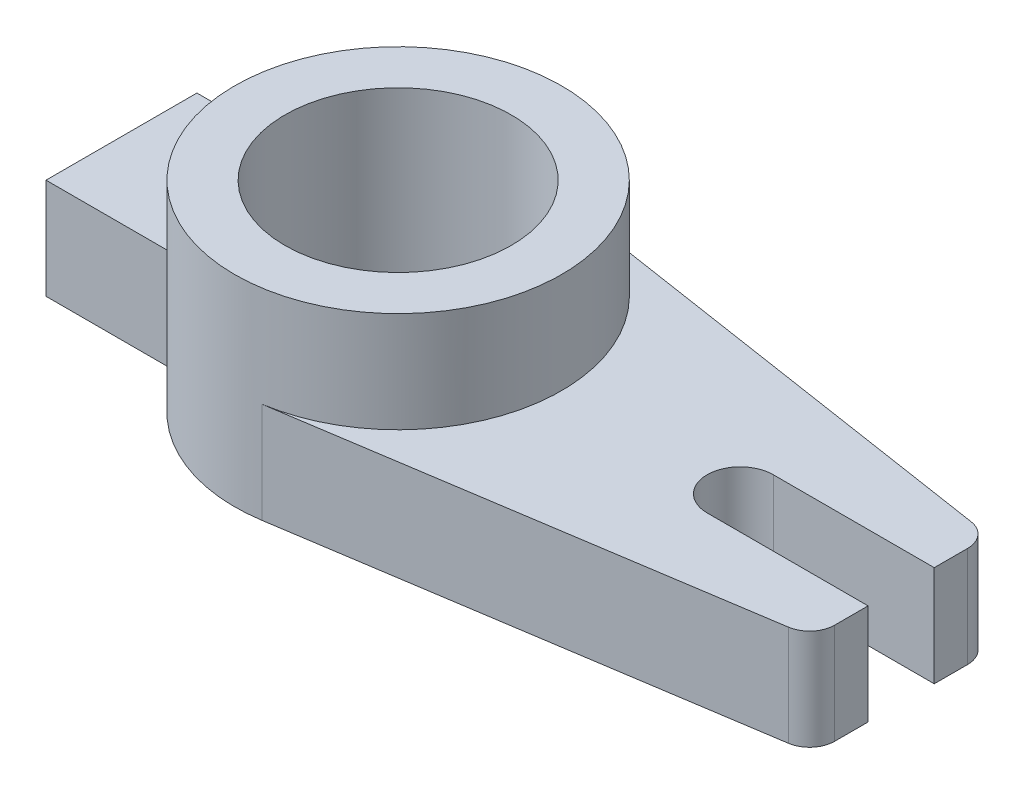
ISO-10303-21;
HEADER;
FILE_DESCRIPTION(('STEP AP214'),'2;1');
FILE_NAME('part.step','',(''),(''),'','','');
FILE_SCHEMA(('AUTOMOTIVE_DESIGN { 1 0 10303 214 1 1 1 1 }'));
ENDSEC;
DATA;
#1=APPLICATION_CONTEXT('core data for automotive mechanical design processes');
#2=APPLICATION_PROTOCOL_DEFINITION('international standard','automotive_design',2000,#1);
#3=PRODUCT_CONTEXT('',#1,'mechanical');
#4=PRODUCT('Part','Part','',(#3));
#5=PRODUCT_RELATED_PRODUCT_CATEGORY('part','',(#4));
#6=PRODUCT_DEFINITION_FORMATION('','',#4);
#7=PRODUCT_DEFINITION_CONTEXT('part definition',#1,'design');
#8=PRODUCT_DEFINITION('design','',#6,#7);
#9=PRODUCT_DEFINITION_SHAPE('','',#8);
#10=(LENGTH_UNIT() NAMED_UNIT(*) SI_UNIT(.MILLI.,.METRE.));
#11=(NAMED_UNIT(*) PLANE_ANGLE_UNIT() SI_UNIT($,.RADIAN.));
#12=(NAMED_UNIT(*) SI_UNIT($,.STERADIAN.) SOLID_ANGLE_UNIT());
#13=UNCERTAINTY_MEASURE_WITH_UNIT(LENGTH_MEASURE(1.E-05),#10,'distance_accuracy_value','');
#14=(GEOMETRIC_REPRESENTATION_CONTEXT(3) GLOBAL_UNCERTAINTY_ASSIGNED_CONTEXT((#13)) GLOBAL_UNIT_ASSIGNED_CONTEXT((#10,
#11,#12)) REPRESENTATION_CONTEXT('',''));
#15=CARTESIAN_POINT('',(0.,0.,0.));
#16=DIRECTION('',(0.,0.,1.));
#17=DIRECTION('',(1.,0.,0.));
#18=AXIS2_PLACEMENT_3D('',#15,#16,#17);
#19=CARTESIAN_POINT('',(0.,40.,0.));
#20=DIRECTION('',(0.,-1.,0.));
#21=DIRECTION('',(0.,0.,-1.));
#22=AXIS2_PLACEMENT_3D('',#19,#20,#21);
#23=CYLINDRICAL_SURFACE('',#22,32.5);
#24=CARTESIAN_POINT('',(0.,40.,0.));
#25=DIRECTION('',(0.,1.,0.));
#26=DIRECTION('',(0.,0.,1.));
#27=AXIS2_PLACEMENT_3D('',#24,#25,#26);
#28=CIRCLE('',#27,32.5);
#29=CARTESIAN_POINT('',(0.,40.,32.5));
#30=VERTEX_POINT('',#29);
#31=EDGE_CURVE('E11',#30,#30,#28,.T.);
#32=ORIENTED_EDGE('',*,*,#31,.F.);
#33=EDGE_LOOP('',(#32));
#34=FACE_BOUND('',#33,.T.);
#35=DIRECTION('',(0.,-1.,0.));
#36=VECTOR('',#35,1.);
#37=CARTESIAN_POINT('',(-28.831406486677,20.,-15.));
#38=LINE('',#37,#36);
#39=CARTESIAN_POINT('',(-28.831406486677,20.,-15.));
#40=VERTEX_POINT('',#39);
#41=CARTESIAN_POINT('',(-28.831406486677,0.,-15.));
#42=VERTEX_POINT('',#41);
#43=EDGE_CURVE('E59',#40,#42,#38,.T.);
#44=ORIENTED_EDGE('',*,*,#43,.F.);
#45=CARTESIAN_POINT('',(0.,20.,0.));
#46=DIRECTION('',(0.,-1.,0.));
#47=DIRECTION('',(0.,0.,1.));
#48=AXIS2_PLACEMENT_3D('',#45,#46,#47);
#49=CIRCLE('',#48,32.5);
#50=CARTESIAN_POINT('',(-28.831406486677,20.,15.));
#51=VERTEX_POINT('',#50);
#52=EDGE_CURVE('E52',#51,#40,#49,.T.);
#53=ORIENTED_EDGE('',*,*,#52,.F.);
#54=DIRECTION('',(0.,-1.,0.));
#55=VECTOR('',#54,1.);
#56=CARTESIAN_POINT('',(-28.831406486677,20.,15.));
#57=LINE('',#56,#55);
#58=CARTESIAN_POINT('',(-28.831406486677,0.,15.));
#59=VERTEX_POINT('',#58);
#60=EDGE_CURVE('E163',#51,#59,#57,.T.);
#61=ORIENTED_EDGE('',*,*,#60,.T.);
#62=CARTESIAN_POINT('',(0.,0.,0.));
#63=DIRECTION('',(0.,1.,0.));
#64=DIRECTION('',(0.,0.,1.));
#65=AXIS2_PLACEMENT_3D('',#62,#63,#64);
#66=CIRCLE('',#65,32.5);
#67=CARTESIAN_POINT('',(5.0678114160152,0.,32.1024498668202));
#68=VERTEX_POINT('',#67);
#69=EDGE_CURVE('E243',#59,#68,#66,.T.);
#70=ORIENTED_EDGE('',*,*,#69,.T.);
#71=DIRECTION('',(0.,-1.,0.));
#72=VECTOR('',#71,1.);
#73=CARTESIAN_POINT('',(5.06781141601827,20.,32.1024498668198));
#74=LINE('',#73,#72);
#75=CARTESIAN_POINT('',(5.06781141601827,20.,32.1024498668197));
#76=VERTEX_POINT('',#75);
#77=EDGE_CURVE('E218',#76,#68,#74,.T.);
#78=ORIENTED_EDGE('',*,*,#77,.F.);
#79=CARTESIAN_POINT('',(0.,20.,0.));
#80=DIRECTION('',(0.,-1.,0.));
#81=DIRECTION('',(0.,0.,1.));
#82=AXIS2_PLACEMENT_3D('',#79,#80,#81);
#83=CIRCLE('',#82,32.5);
#84=CARTESIAN_POINT('',(5.0678114160152,20.,-32.1024498668202));
#85=VERTEX_POINT('',#84);
#86=EDGE_CURVE('E182',#85,#76,#83,.T.);
#87=ORIENTED_EDGE('',*,*,#86,.F.);
#88=DIRECTION('',(0.,-1.,0.));
#89=VECTOR('',#88,1.);
#90=CARTESIAN_POINT('',(5.06781141601827,20.,-32.1024498668198));
#91=LINE('',#90,#89);
#92=CARTESIAN_POINT('',(5.06781141601827,0.,-32.1024498668198));
#93=VERTEX_POINT('',#92);
#94=EDGE_CURVE('E225',#85,#93,#91,.T.);
#95=ORIENTED_EDGE('',*,*,#94,.T.);
#96=EDGE_CURVE('E45',#93,#42,#66,.T.);
#97=ORIENTED_EDGE('',*,*,#96,.T.);
#98=EDGE_LOOP('',(#44,#53,#61,#70,#78,#87,#95,#97));
#99=FACE_BOUND('',#98,.T.);
#100=ADVANCED_FACE('F39',(#34,#99),#23,.T.);
#101=CARTESIAN_POINT('',(0.,40.,0.));
#102=DIRECTION('',(0.,1.,0.));
#103=DIRECTION('',(0.,0.,1.));
#104=AXIS2_PLACEMENT_3D('',#101,#102,#103);
#105=PLANE('',#104);
#106=ORIENTED_EDGE('',*,*,#31,.T.);
#107=EDGE_LOOP('',(#106));
#108=FACE_BOUND('',#107,.T.);
#109=CARTESIAN_POINT('',(0.,40.,0.));
#110=DIRECTION('',(0.,1.,0.));
#111=DIRECTION('',(0.,0.,1.));
#112=AXIS2_PLACEMENT_3D('',#109,#110,#111);
#113=CIRCLE('',#112,22.5);
#114=CARTESIAN_POINT('',(0.,40.,22.5));
#115=VERTEX_POINT('',#114);
#116=EDGE_CURVE('E236',#115,#115,#113,.T.);
#117=ORIENTED_EDGE('',*,*,#116,.F.);
#118=EDGE_LOOP('',(#117));
#119=FACE_BOUND('',#118,.T.);
#120=ADVANCED_FACE('F257',(#108,#119),#105,.T.);
#121=CARTESIAN_POINT('',(0.,0.,0.));
#122=DIRECTION('',(0.,1.,0.));
#123=DIRECTION('',(0.,0.,1.));
#124=AXIS2_PLACEMENT_3D('',#121,#122,#123);
#125=PLANE('',#124);
#126=ORIENTED_EDGE('',*,*,#96,.F.);
#127=DIRECTION('',(-0.988375612593621,0.,-0.152031734944335));
#128=VECTOR('',#127,1.);
#129=CARTESIAN_POINT('',(95.7601586747217,0.,-18.1521715270567));
#130=LINE('',#129,#128);
#131=CARTESIAN_POINT('',(95.7601586747217,0.,-18.1521715270567));
#132=VERTEX_POINT('',#131);
#133=EDGE_CURVE('E196',#132,#93,#130,.T.);
#134=ORIENTED_EDGE('',*,*,#133,.F.);
#135=CARTESIAN_POINT('',(95.,0.,-13.2102934640886));
#136=DIRECTION('',(0.,1.,0.));
#137=DIRECTION('',(0.,0.,1.));
#138=AXIS2_PLACEMENT_3D('',#135,#136,#137);
#139=CIRCLE('',#138,5.);
#140=CARTESIAN_POINT('',(100.,0.,-13.2102934640886));
#141=VERTEX_POINT('',#140);
#142=EDGE_CURVE('E198',#141,#132,#139,.T.);
#143=ORIENTED_EDGE('',*,*,#142,.F.);
#144=DIRECTION('',(0.,0.,-1.));
#145=VECTOR('',#144,1.);
#146=CARTESIAN_POINT('',(100.,0.,-6.57658921600583));
#147=LINE('',#146,#145);
#148=CARTESIAN_POINT('',(100.,0.,-6.57658921600583));
#149=VERTEX_POINT('',#148);
#150=EDGE_CURVE('E192',#149,#141,#147,.T.);
#151=ORIENTED_EDGE('',*,*,#150,.F.);
#152=DIRECTION('',(1.,0.,0.));
#153=VECTOR('',#152,1.);
#154=CARTESIAN_POINT('',(68.,0.,-6.57658921600583));
#155=LINE('',#154,#153);
#156=CARTESIAN_POINT('',(68.,0.,-6.57658921600583));
#157=VERTEX_POINT('',#156);
#158=EDGE_CURVE('E165',#157,#149,#155,.T.);
#159=ORIENTED_EDGE('',*,*,#158,.F.);
#160=CARTESIAN_POINT('',(68.,0.,0.));
#161=DIRECTION('',(0.,-1.,0.));
#162=DIRECTION('',(0.,0.,1.));
#163=AXIS2_PLACEMENT_3D('',#160,#161,#162);
#164=CIRCLE('',#163,6.57658921600583);
#165=CARTESIAN_POINT('',(68.,0.,6.57658921600583));
#166=VERTEX_POINT('',#165);
#167=EDGE_CURVE('E157',#166,#157,#164,.T.);
#168=ORIENTED_EDGE('',*,*,#167,.F.);
#169=DIRECTION('',(-1.,0.,0.));
#170=VECTOR('',#169,1.);
#171=CARTESIAN_POINT('',(68.,0.,6.57658921600583));
#172=LINE('',#171,#170);
#173=CARTESIAN_POINT('',(100.,0.,6.57658921600583));
#174=VERTEX_POINT('',#173);
#175=EDGE_CURVE('E174',#174,#166,#172,.T.);
#176=ORIENTED_EDGE('',*,*,#175,.F.);
#177=DIRECTION('',(0.,0.,-1.));
#178=VECTOR('',#177,1.);
#179=CARTESIAN_POINT('',(100.,0.,6.57658921600583));
#180=LINE('',#179,#178);
#181=CARTESIAN_POINT('',(100.,0.,13.2102934640886));
#182=VERTEX_POINT('',#181);
#183=EDGE_CURVE('E202',#182,#174,#180,.T.);
#184=ORIENTED_EDGE('',*,*,#183,.F.);
#185=CARTESIAN_POINT('',(95.,0.,13.2102934640886));
#186=DIRECTION('',(0.,1.,0.));
#187=DIRECTION('',(0.,0.,1.));
#188=AXIS2_PLACEMENT_3D('',#185,#186,#187);
#189=CIRCLE('',#188,5.);
#190=CARTESIAN_POINT('',(95.7601586747217,0.,18.1521715270567));
#191=VERTEX_POINT('',#190);
#192=EDGE_CURVE('E201',#191,#182,#189,.T.);
#193=ORIENTED_EDGE('',*,*,#192,.F.);
#194=DIRECTION('',(0.988375612593621,0.,-0.152031734944335));
#195=VECTOR('',#194,1.);
#196=CARTESIAN_POINT('',(95.7601586747217,0.,18.1521715270567));
#197=LINE('',#196,#195);
#198=EDGE_CURVE('E203',#68,#191,#197,.T.);
#199=ORIENTED_EDGE('',*,*,#198,.F.);
#200=ORIENTED_EDGE('',*,*,#69,.F.);
#201=DIRECTION('',(1.,0.,0.));
#202=VECTOR('',#201,1.);
#203=CARTESIAN_POINT('',(-28.831406486677,0.,15.));
#204=LINE('',#203,#202);
#205=CARTESIAN_POINT('',(-55.,0.,15.));
#206=VERTEX_POINT('',#205);
#207=EDGE_CURVE('E152',#206,#59,#204,.T.);
#208=ORIENTED_EDGE('',*,*,#207,.F.);
#209=DIRECTION('',(0.,0.,1.));
#210=VECTOR('',#209,1.);
#211=CARTESIAN_POINT('',(-55.,0.,15.));
#212=LINE('',#211,#210);
#213=CARTESIAN_POINT('',(-55.,0.,-15.));
#214=VERTEX_POINT('',#213);
#215=EDGE_CURVE('E420',#214,#206,#212,.T.);
#216=ORIENTED_EDGE('',*,*,#215,.F.);
#217=DIRECTION('',(-1.,0.,0.));
#218=VECTOR('',#217,1.);
#219=CARTESIAN_POINT('',(-55.,0.,-15.));
#220=LINE('',#219,#218);
#221=EDGE_CURVE('E158',#42,#214,#220,.T.);
#222=ORIENTED_EDGE('',*,*,#221,.F.);
#223=EDGE_LOOP('',(#126,#134,#143,#151,#159,#168,#176,#184,#193,#199,#200,#208,#216,#222));
#224=FACE_BOUND('',#223,.T.);
#225=CARTESIAN_POINT('',(0.,0.,0.));
#226=DIRECTION('',(0.,1.,0.));
#227=DIRECTION('',(0.,0.,1.));
#228=AXIS2_PLACEMENT_3D('',#225,#226,#227);
#229=CIRCLE('',#228,22.5);
#230=CARTESIAN_POINT('',(0.,0.,22.5));
#231=VERTEX_POINT('',#230);
#232=EDGE_CURVE('E240',#231,#231,#229,.T.);
#233=ORIENTED_EDGE('',*,*,#232,.T.);
#234=EDGE_LOOP('',(#233));
#235=FACE_BOUND('',#234,.T.);
#236=ADVANCED_FACE('F241',(#224,#235),#125,.F.);
#237=CARTESIAN_POINT('',(0.,40.,0.));
#238=DIRECTION('',(0.,-1.,0.));
#239=DIRECTION('',(0.,0.,-1.));
#240=AXIS2_PLACEMENT_3D('',#237,#238,#239);
#241=CYLINDRICAL_SURFACE('',#240,22.5);
#242=ORIENTED_EDGE('',*,*,#116,.T.);
#243=EDGE_LOOP('',(#242));
#244=FACE_BOUND('',#243,.T.);
#245=ORIENTED_EDGE('',*,*,#232,.F.);
#246=EDGE_LOOP('',(#245));
#247=FACE_BOUND('',#246,.T.);
#248=ADVANCED_FACE('F250',(#244,#247),#241,.F.);
#249=CARTESIAN_POINT('',(68.,20.,0.));
#250=DIRECTION('',(0.,-1.,0.));
#251=DIRECTION('',(0.,0.,-1.));
#252=AXIS2_PLACEMENT_3D('',#249,#250,#251);
#253=CYLINDRICAL_SURFACE('',#252,6.57658921600583);
#254=ORIENTED_EDGE('',*,*,#167,.T.);
#255=DIRECTION('',(0.,-1.,0.));
#256=VECTOR('',#255,1.);
#257=CARTESIAN_POINT('',(68.,20.,-6.57658921600583));
#258=LINE('',#257,#256);
#259=CARTESIAN_POINT('',(68.,20.,-6.57658921600583));
#260=VERTEX_POINT('',#259);
#261=EDGE_CURVE('E232',#260,#157,#258,.T.);
#262=ORIENTED_EDGE('',*,*,#261,.F.);
#263=CARTESIAN_POINT('',(68.,20.,0.));
#264=DIRECTION('',(0.,-1.,0.));
#265=DIRECTION('',(0.,0.,1.));
#266=AXIS2_PLACEMENT_3D('',#263,#264,#265);
#267=CIRCLE('',#266,6.57658921600583);
#268=CARTESIAN_POINT('',(68.,20.,6.57658921600583));
#269=VERTEX_POINT('',#268);
#270=EDGE_CURVE('E169',#269,#260,#267,.T.);
#271=ORIENTED_EDGE('',*,*,#270,.F.);
#272=DIRECTION('',(0.,-1.,0.));
#273=VECTOR('',#272,1.);
#274=CARTESIAN_POINT('',(68.,20.,6.57658921600583));
#275=LINE('',#274,#273);
#276=EDGE_CURVE('E193',#269,#166,#275,.T.);
#277=ORIENTED_EDGE('',*,*,#276,.T.);
#278=EDGE_LOOP('',(#254,#262,#271,#277));
#279=FACE_BOUND('',#278,.T.);
#280=ADVANCED_FACE('F247',(#279),#253,.F.);
#281=CARTESIAN_POINT('',(68.,20.,-6.57658921600583));
#282=DIRECTION('',(0.,0.,-1.));
#283=DIRECTION('',(-1.,0.,0.));
#284=AXIS2_PLACEMENT_3D('',#281,#282,#283);
#285=PLANE('',#284);
#286=ORIENTED_EDGE('',*,*,#158,.T.);
#287=DIRECTION('',(0.,-1.,0.));
#288=VECTOR('',#287,1.);
#289=CARTESIAN_POINT('',(100.,20.,-6.57658921600583));
#290=LINE('',#289,#288);
#291=CARTESIAN_POINT('',(100.,20.,-6.57658921600583));
#292=VERTEX_POINT('',#291);
#293=EDGE_CURVE('E233',#292,#149,#290,.T.);
#294=ORIENTED_EDGE('',*,*,#293,.F.);
#295=DIRECTION('',(1.,0.,0.));
#296=VECTOR('',#295,1.);
#297=CARTESIAN_POINT('',(68.,20.,-6.57658921600583));
#298=LINE('',#297,#296);
#299=EDGE_CURVE('E173',#260,#292,#298,.T.);
#300=ORIENTED_EDGE('',*,*,#299,.F.);
#301=ORIENTED_EDGE('',*,*,#261,.T.);
#302=EDGE_LOOP('',(#286,#294,#300,#301));
#303=FACE_BOUND('',#302,.T.);
#304=ADVANCED_FACE('F258',(#303),#285,.F.);
#305=CARTESIAN_POINT('',(100.,20.,-6.57658921600583));
#306=DIRECTION('',(-1.,0.,0.));
#307=DIRECTION('',(0.,0.,1.));
#308=AXIS2_PLACEMENT_3D('',#305,#306,#307);
#309=PLANE('',#308);
#310=ORIENTED_EDGE('',*,*,#150,.T.);
#311=DIRECTION('',(0.,-1.,0.));
#312=VECTOR('',#311,1.);
#313=CARTESIAN_POINT('',(100.,20.,-13.2102934640886));
#314=LINE('',#313,#312);
#315=CARTESIAN_POINT('',(100.,20.,-13.2102934640886));
#316=VERTEX_POINT('',#315);
#317=EDGE_CURVE('E227',#316,#141,#314,.T.);
#318=ORIENTED_EDGE('',*,*,#317,.F.);
#319=DIRECTION('',(0.,0.,-1.));
#320=VECTOR('',#319,1.);
#321=CARTESIAN_POINT('',(100.,20.,-6.57658921600583));
#322=LINE('',#321,#320);
#323=EDGE_CURVE('E175',#292,#316,#322,.T.);
#324=ORIENTED_EDGE('',*,*,#323,.F.);
#325=ORIENTED_EDGE('',*,*,#293,.T.);
#326=EDGE_LOOP('',(#310,#318,#324,#325));
#327=FACE_BOUND('',#326,.T.);
#328=ADVANCED_FACE('F303',(#327),#309,.F.);
#329=CARTESIAN_POINT('',(95.,20.,-13.2102934640886));
#330=DIRECTION('',(0.,-1.,0.));
#331=DIRECTION('',(0.,0.,-1.));
#332=AXIS2_PLACEMENT_3D('',#329,#330,#331);
#333=CYLINDRICAL_SURFACE('',#332,5.);
#334=ORIENTED_EDGE('',*,*,#142,.T.);
#335=DIRECTION('',(0.,-1.,0.));
#336=VECTOR('',#335,1.);
#337=CARTESIAN_POINT('',(95.7601586747217,20.,-18.1521715270567));
#338=LINE('',#337,#336);
#339=CARTESIAN_POINT('',(95.7601586747217,20.,-18.1521715270567));
#340=VERTEX_POINT('',#339);
#341=EDGE_CURVE('E223',#340,#132,#338,.T.);
#342=ORIENTED_EDGE('',*,*,#341,.F.);
#343=CARTESIAN_POINT('',(95.,20.,-13.2102934640886));
#344=DIRECTION('',(0.,1.,0.));
#345=DIRECTION('',(0.,0.,1.));
#346=AXIS2_PLACEMENT_3D('',#343,#344,#345);
#347=CIRCLE('',#346,5.);
#348=EDGE_CURVE('E178',#316,#340,#347,.T.);
#349=ORIENTED_EDGE('',*,*,#348,.F.);
#350=ORIENTED_EDGE('',*,*,#317,.T.);
#351=EDGE_LOOP('',(#334,#342,#349,#350));
#352=FACE_BOUND('',#351,.T.);
#353=ADVANCED_FACE('F309',(#352),#333,.T.);
#354=CARTESIAN_POINT('',(95.7601586747217,20.,-18.1521715270567));
#355=DIRECTION('',(-0.152031734944335,0.,0.988375612593621));
#356=DIRECTION('',(0.988375612593621,0.,0.152031734944335));
#357=AXIS2_PLACEMENT_3D('',#354,#355,#356);
#358=PLANE('',#357);
#359=ORIENTED_EDGE('',*,*,#133,.T.);
#360=ORIENTED_EDGE('',*,*,#94,.F.);
#361=DIRECTION('',(-0.988375612593621,0.,-0.152031734944335));
#362=VECTOR('',#361,1.);
#363=CARTESIAN_POINT('',(95.7601586747217,20.,-18.1521715270567));
#364=LINE('',#363,#362);
#365=EDGE_CURVE('E176',#340,#85,#364,.T.);
#366=ORIENTED_EDGE('',*,*,#365,.F.);
#367=ORIENTED_EDGE('',*,*,#341,.T.);
#368=EDGE_LOOP('',(#359,#360,#366,#367));
#369=FACE_BOUND('',#368,.T.);
#370=ADVANCED_FACE('F317',(#369),#358,.F.);
#371=CARTESIAN_POINT('',(95.7601586747217,20.,18.1521715270567));
#372=DIRECTION('',(-0.152031734944335,0.,-0.988375612593621));
#373=DIRECTION('',(-0.988375612593621,0.,0.152031734944335));
#374=AXIS2_PLACEMENT_3D('',#371,#372,#373);
#375=PLANE('',#374);
#376=ORIENTED_EDGE('',*,*,#198,.T.);
#377=DIRECTION('',(0.,-1.,0.));
#378=VECTOR('',#377,1.);
#379=CARTESIAN_POINT('',(95.7601586747217,20.,18.1521715270567));
#380=LINE('',#379,#378);
#381=CARTESIAN_POINT('',(95.7601586747217,20.,18.1521715270567));
#382=VERTEX_POINT('',#381);
#383=EDGE_CURVE('E216',#382,#191,#380,.T.);
#384=ORIENTED_EDGE('',*,*,#383,.F.);
#385=DIRECTION('',(0.988375612593621,0.,-0.152031734944335));
#386=VECTOR('',#385,1.);
#387=CARTESIAN_POINT('',(95.7601586747217,20.,18.1521715270567));
#388=LINE('',#387,#386);
#389=EDGE_CURVE('E184',#76,#382,#388,.T.);
#390=ORIENTED_EDGE('',*,*,#389,.F.);
#391=ORIENTED_EDGE('',*,*,#77,.T.);
#392=EDGE_LOOP('',(#376,#384,#390,#391));
#393=FACE_BOUND('',#392,.T.);
#394=ADVANCED_FACE('F327',(#393),#375,.F.);
#395=CARTESIAN_POINT('',(95.,20.,13.2102934640886));
#396=DIRECTION('',(0.,-1.,0.));
#397=DIRECTION('',(0.,0.,-1.));
#398=AXIS2_PLACEMENT_3D('',#395,#396,#397);
#399=CYLINDRICAL_SURFACE('',#398,5.);
#400=ORIENTED_EDGE('',*,*,#192,.T.);
#401=DIRECTION('',(0.,-1.,0.));
#402=VECTOR('',#401,1.);
#403=CARTESIAN_POINT('',(100.,20.,13.2102934640886));
#404=LINE('',#403,#402);
#405=CARTESIAN_POINT('',(100.,20.,13.2102934640886));
#406=VERTEX_POINT('',#405);
#407=EDGE_CURVE('E213',#406,#182,#404,.T.);
#408=ORIENTED_EDGE('',*,*,#407,.F.);
#409=CARTESIAN_POINT('',(95.,20.,13.2102934640886));
#410=DIRECTION('',(0.,1.,0.));
#411=DIRECTION('',(0.,0.,1.));
#412=AXIS2_PLACEMENT_3D('',#409,#410,#411);
#413=CIRCLE('',#412,5.);
#414=EDGE_CURVE('E188',#382,#406,#413,.T.);
#415=ORIENTED_EDGE('',*,*,#414,.F.);
#416=ORIENTED_EDGE('',*,*,#383,.T.);
#417=EDGE_LOOP('',(#400,#408,#415,#416));
#418=FACE_BOUND('',#417,.T.);
#419=ADVANCED_FACE('F339',(#418),#399,.T.);
#420=CARTESIAN_POINT('',(100.,20.,6.57658921600583));
#421=DIRECTION('',(-1.,0.,0.));
#422=DIRECTION('',(0.,0.,1.));
#423=AXIS2_PLACEMENT_3D('',#420,#421,#422);
#424=PLANE('',#423);
#425=ORIENTED_EDGE('',*,*,#183,.T.);
#426=DIRECTION('',(0.,-1.,0.));
#427=VECTOR('',#426,1.);
#428=CARTESIAN_POINT('',(100.,20.,6.57658921600583));
#429=LINE('',#428,#427);
#430=CARTESIAN_POINT('',(100.,20.,6.57658921600583));
#431=VERTEX_POINT('',#430);
#432=EDGE_CURVE('E209',#431,#174,#429,.T.);
#433=ORIENTED_EDGE('',*,*,#432,.F.);
#434=DIRECTION('',(0.,0.,-1.));
#435=VECTOR('',#434,1.);
#436=CARTESIAN_POINT('',(100.,20.,6.57658921600583));
#437=LINE('',#436,#435);
#438=EDGE_CURVE('E187',#406,#431,#437,.T.);
#439=ORIENTED_EDGE('',*,*,#438,.F.);
#440=ORIENTED_EDGE('',*,*,#407,.T.);
#441=EDGE_LOOP('',(#425,#433,#439,#440));
#442=FACE_BOUND('',#441,.T.);
#443=ADVANCED_FACE('F347',(#442),#424,.F.);
#444=CARTESIAN_POINT('',(68.,20.,6.57658921600583));
#445=DIRECTION('',(0.,0.,1.));
#446=DIRECTION('',(1.,0.,0.));
#447=AXIS2_PLACEMENT_3D('',#444,#445,#446);
#448=PLANE('',#447);
#449=ORIENTED_EDGE('',*,*,#175,.T.);
#450=ORIENTED_EDGE('',*,*,#276,.F.);
#451=DIRECTION('',(-1.,0.,0.));
#452=VECTOR('',#451,1.);
#453=CARTESIAN_POINT('',(68.,20.,6.57658921600583));
#454=LINE('',#453,#452);
#455=EDGE_CURVE('E186',#431,#269,#454,.T.);
#456=ORIENTED_EDGE('',*,*,#455,.F.);
#457=ORIENTED_EDGE('',*,*,#432,.T.);
#458=EDGE_LOOP('',(#449,#450,#456,#457));
#459=FACE_BOUND('',#458,.T.);
#460=ADVANCED_FACE('F351',(#459),#448,.F.);
#461=CARTESIAN_POINT('',(68.,20.,0.));
#462=DIRECTION('',(0.,1.,0.));
#463=DIRECTION('',(0.,0.,1.));
#464=AXIS2_PLACEMENT_3D('',#461,#462,#463);
#465=PLANE('',#464);
#466=ORIENTED_EDGE('',*,*,#270,.T.);
#467=ORIENTED_EDGE('',*,*,#299,.T.);
#468=ORIENTED_EDGE('',*,*,#323,.T.);
#469=ORIENTED_EDGE('',*,*,#348,.T.);
#470=ORIENTED_EDGE('',*,*,#365,.T.);
#471=ORIENTED_EDGE('',*,*,#86,.T.);
#472=ORIENTED_EDGE('',*,*,#389,.T.);
#473=ORIENTED_EDGE('',*,*,#414,.T.);
#474=ORIENTED_EDGE('',*,*,#438,.T.);
#475=ORIENTED_EDGE('',*,*,#455,.T.);
#476=EDGE_LOOP('',(#466,#467,#468,#469,#470,#471,#472,#473,#474,#475));
#477=FACE_BOUND('',#476,.T.);
#478=ADVANCED_FACE('F365',(#477),#465,.T.);
#479=CARTESIAN_POINT('',(-55.,20.,-15.));
#480=DIRECTION('',(0.,0.,1.));
#481=DIRECTION('',(1.,0.,0.));
#482=AXIS2_PLACEMENT_3D('',#479,#480,#481);
#483=PLANE('',#482);
#484=ORIENTED_EDGE('',*,*,#221,.T.);
#485=DIRECTION('',(0.,-1.,0.));
#486=VECTOR('',#485,1.);
#487=CARTESIAN_POINT('',(-55.,20.,-15.));
#488=LINE('',#487,#486);
#489=CARTESIAN_POINT('',(-55.,20.,-15.));
#490=VERTEX_POINT('',#489);
#491=EDGE_CURVE('E142',#490,#214,#488,.T.);
#492=ORIENTED_EDGE('',*,*,#491,.F.);
#493=DIRECTION('',(-1.,0.,0.));
#494=VECTOR('',#493,1.);
#495=CARTESIAN_POINT('',(-55.,20.,-15.));
#496=LINE('',#495,#494);
#497=EDGE_CURVE('E149',#40,#490,#496,.T.);
#498=ORIENTED_EDGE('',*,*,#497,.F.);
#499=ORIENTED_EDGE('',*,*,#43,.T.);
#500=EDGE_LOOP('',(#484,#492,#498,#499));
#501=FACE_BOUND('',#500,.T.);
#502=ADVANCED_FACE('F156',(#501),#483,.F.);
#503=CARTESIAN_POINT('',(-55.,20.,15.));
#504=DIRECTION('',(1.,0.,0.));
#505=DIRECTION('',(0.,0.,-1.));
#506=AXIS2_PLACEMENT_3D('',#503,#504,#505);
#507=PLANE('',#506);
#508=ORIENTED_EDGE('',*,*,#215,.T.);
#509=DIRECTION('',(0.,-1.,0.));
#510=VECTOR('',#509,1.);
#511=CARTESIAN_POINT('',(-55.,20.,15.));
#512=LINE('',#511,#510);
#513=CARTESIAN_POINT('',(-55.,20.,15.));
#514=VERTEX_POINT('',#513);
#515=EDGE_CURVE('E144',#514,#206,#512,.T.);
#516=ORIENTED_EDGE('',*,*,#515,.F.);
#517=DIRECTION('',(0.,0.,1.));
#518=VECTOR('',#517,1.);
#519=CARTESIAN_POINT('',(-55.,20.,15.));
#520=LINE('',#519,#518);
#521=EDGE_CURVE('E136',#490,#514,#520,.T.);
#522=ORIENTED_EDGE('',*,*,#521,.F.);
#523=ORIENTED_EDGE('',*,*,#491,.T.);
#524=EDGE_LOOP('',(#508,#516,#522,#523));
#525=FACE_BOUND('',#524,.T.);
#526=ADVANCED_FACE('F139',(#525),#507,.F.);
#527=CARTESIAN_POINT('',(-28.831406486677,20.,15.));
#528=DIRECTION('',(0.,0.,-1.));
#529=DIRECTION('',(-1.,0.,0.));
#530=AXIS2_PLACEMENT_3D('',#527,#528,#529);
#531=PLANE('',#530);
#532=ORIENTED_EDGE('',*,*,#207,.T.);
#533=ORIENTED_EDGE('',*,*,#60,.F.);
#534=DIRECTION('',(1.,0.,0.));
#535=VECTOR('',#534,1.);
#536=CARTESIAN_POINT('',(-28.831406486677,20.,15.));
#537=LINE('',#536,#535);
#538=EDGE_CURVE('E146',#514,#51,#537,.T.);
#539=ORIENTED_EDGE('',*,*,#538,.F.);
#540=ORIENTED_EDGE('',*,*,#515,.T.);
#541=EDGE_LOOP('',(#532,#533,#539,#540));
#542=FACE_BOUND('',#541,.T.);
#543=ADVANCED_FACE('F393',(#542),#531,.F.);
#544=CARTESIAN_POINT('',(0.,20.,0.));
#545=DIRECTION('',(0.,1.,0.));
#546=DIRECTION('',(0.,0.,1.));
#547=AXIS2_PLACEMENT_3D('',#544,#545,#546);
#548=PLANE('',#547);
#549=ORIENTED_EDGE('',*,*,#497,.T.);
#550=ORIENTED_EDGE('',*,*,#521,.T.);
#551=ORIENTED_EDGE('',*,*,#538,.T.);
#552=ORIENTED_EDGE('',*,*,#52,.T.);
#553=EDGE_LOOP('',(#549,#550,#551,#552));
#554=FACE_BOUND('',#553,.T.);
#555=ADVANCED_FACE('F155',(#554),#548,.T.);
#556=CLOSED_SHELL('',(#100,#120,#236,#248,#280,#304,#328,#353,#370,#394,#419,#443,#460,#478,
#502,#526,#543,#555));
#557=MANIFOLD_SOLID_BREP('B2',#556);
#558=ADVANCED_BREP_SHAPE_REPRESENTATION('',(#18,#557),#14);
#559=SHAPE_DEFINITION_REPRESENTATION(#9,#558);
ENDSEC;
END-ISO-10303-21;
